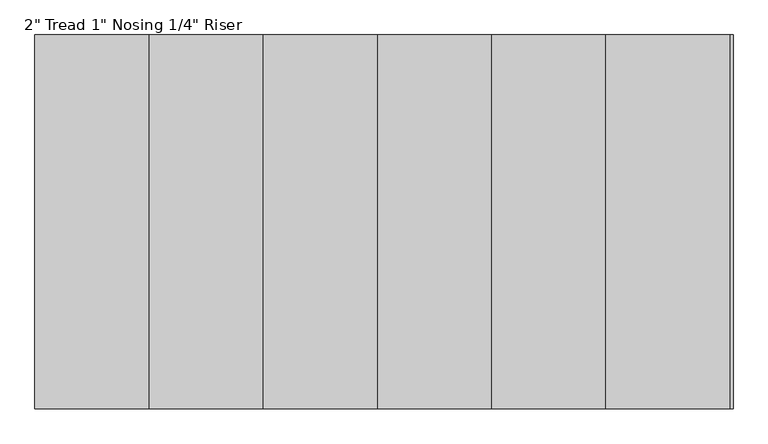
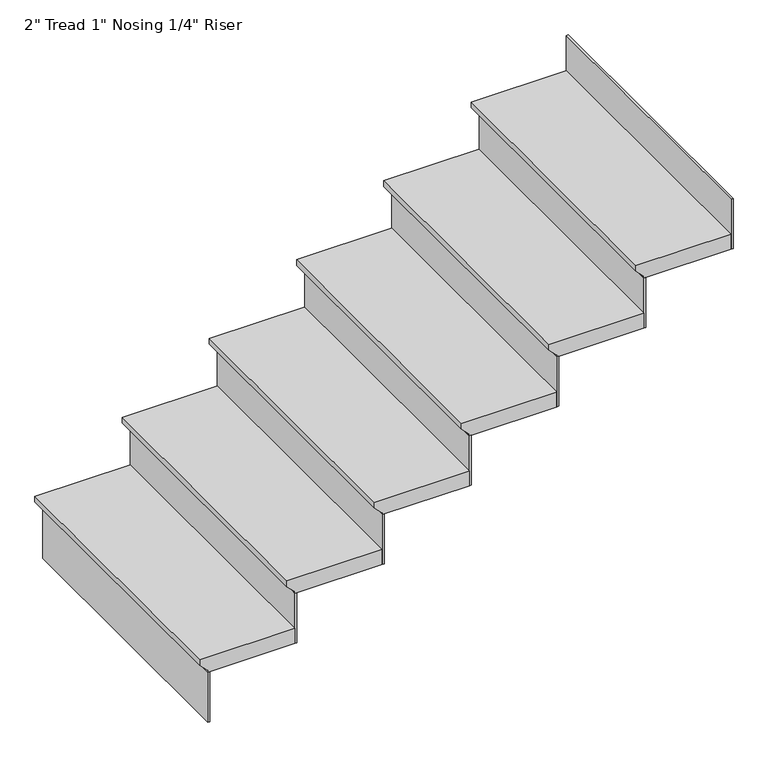
"""IFC4 building model written with IfcOpenShell, lengths in millimetres: stair flight geometry."""

from ifc_helpers import new_model, si_unit, frame, origin, place, context, project, spatial, polyline, outline, extrude, source, transform, mapped, element, save


def stair_flight_86d1b198(model_context):
    return source(origin(), model_context, "Body", "SweptSolid", [
        extrude(outline(polyline([(2336.8, -8480.0517085), (2336.8, -8784.8517085), (2317.75, -8784.8517085), (2292.35, -8759.4517085), (2286.0, -8759.4517085), (2286.0, -8480.0517085), (2336.8, -8480.0517085)])), frame((0.0, 792.0165128, 0.0), z_axis=(0.0, 1.0, 0.0), x_axis=(0.0, 0.0, 1.0)), (0.0, 0.0, 1.0), 914.4),
        extrude(outline(polyline([(-8753.1017085, 792.0165128), (-8759.4517085, 792.0165128), (-8759.4517085, 1706.4165128), (-8753.1017085, 1706.4165128), (-8753.1017085, 792.0165128)])), frame((0.0, 0.0, 2116.6666667), z_axis=(0.0, 0.0, 1.0), x_axis=(1.0, 0.0, 0.0)), (0.0, 0.0, 1.0), 169.3333333),
        extrude(outline(polyline([(-8473.7017085, 792.0165128), (-8480.0517085, 792.0165128), (-8480.0517085, 1706.4165128), (-8473.7017085, 1706.4165128), (-8473.7017085, 792.0165128)])), frame((0.0, 0.0, 2286.0), z_axis=(0.0, 0.0, 1.0), x_axis=(1.0, 0.0, 0.0)), (0.0, 0.0, 1.0), 169.3333333),
        extrude(outline(polyline([(2506.1333333, -8200.6517085), (2506.1333333, -8505.4517085), (2487.0833333, -8505.4517085), (2461.6833333, -8480.0517085), (2455.3333333, -8480.0517085), (2455.3333333, -8200.6517085), (2506.1333333, -8200.6517085)])), frame((0.0, 792.0165128, 0.0), z_axis=(0.0, 1.0, 0.0), x_axis=(0.0, 0.0, 1.0)), (0.0, 0.0, 1.0), 914.4),
        extrude(outline(polyline([(-8194.3017085, 792.0165128), (-8200.6517085, 792.0165128), (-8200.6517085, 1706.4165128), (-8194.3017085, 1706.4165128), (-8194.3017085, 792.0165128)])), frame((0.0, 0.0, 2455.3333333), z_axis=(0.0, 0.0, 1.0), x_axis=(1.0, 0.0, 0.0)), (0.0, 0.0, 1.0), 169.3333333),
        extrude(outline(polyline([(2675.4666667, -7921.2517085), (2675.4666667, -8226.0517085), (2656.4166667, -8226.0517085), (2631.0166667, -8200.6517085), (2624.6666667, -8200.6517085), (2624.6666667, -7921.2517085), (2675.4666667, -7921.2517085)])), frame((0.0, 792.0165128, 0.0), z_axis=(0.0, 1.0, 0.0), x_axis=(0.0, 0.0, 1.0)), (0.0, 0.0, 1.0), 914.4),
        extrude(outline(polyline([(-7914.9017085, 792.0165128), (-7921.2517085, 792.0165128), (-7921.2517085, 1706.4165128), (-7914.9017085, 1706.4165128), (-7914.9017085, 792.0165128)])), frame((0.0, 0.0, 2624.6666667), z_axis=(0.0, 0.0, 1.0), x_axis=(1.0, 0.0, 0.0)), (0.0, 0.0, 1.0), 169.3333333),
        extrude(outline(polyline([(2844.8, -7641.8517085), (2844.8, -7946.6517085), (2825.75, -7946.6517085), (2800.35, -7921.2517085), (2794.0, -7921.2517085), (2794.0, -7641.8517085), (2844.8, -7641.8517085)])), frame((0.0, 792.0165128, 0.0), z_axis=(0.0, 1.0, 0.0), x_axis=(0.0, 0.0, 1.0)), (0.0, 0.0, 1.0), 914.4),
        extrude(outline(polyline([(-7635.5017085, 792.0165128), (-7641.8517085, 792.0165128), (-7641.8517085, 1706.4165128), (-7635.5017085, 1706.4165128), (-7635.5017085, 792.0165128)])), frame((0.0, 0.0, 2794.0), z_axis=(0.0, 0.0, 1.0), x_axis=(1.0, 0.0, 0.0)), (0.0, 0.0, 1.0), 169.3333333),
        extrude(outline(polyline([(3014.1333333, -7362.4517085), (3014.1333333, -7667.2517085), (2995.0833333, -7667.2517085), (2969.6833333, -7641.8517085), (2963.3333333, -7641.8517085), (2963.3333333, -7362.4517085), (3014.1333333, -7362.4517085)])), frame((0.0, 792.0165128, 0.0), z_axis=(0.0, 1.0, 0.0), x_axis=(0.0, 0.0, 1.0)), (0.0, 0.0, 1.0), 914.4),
        extrude(outline(polyline([(-7356.1017085, 792.0165128), (-7362.4517085, 792.0165128), (-7362.4517085, 1706.4165128), (-7356.1017085, 1706.4165128), (-7356.1017085, 792.0165128)])), frame((0.0, 0.0, 2963.3333333), z_axis=(0.0, 0.0, 1.0), x_axis=(1.0, 0.0, 0.0)), (0.0, 0.0, 1.0), 169.3333333),
        extrude(outline(polyline([(-7076.7017085, 792.0165128), (-7083.0517085, 792.0165128), (-7083.0517085, 1706.4165128), (-7076.7017085, 1706.4165128), (-7076.7017085, 792.0165128)])), frame((0.0, 0.0, 3132.6666667), z_axis=(0.0, 0.0, 1.0), x_axis=(1.0, 0.0, 0.0)), (0.0, 0.0, 1.0), 169.3333333),
        extrude(outline(polyline([(3183.4666667, -7083.0517085), (3183.4666667, -7387.8517085), (3164.4166667, -7387.8517085), (3139.0166667, -7362.4517085), (3132.6666667, -7362.4517085), (3132.6666667, -7083.0517085), (3183.4666667, -7083.0517085)])), frame((0.0, 792.0165128, 0.0), z_axis=(0.0, 1.0, 0.0), x_axis=(0.0, 0.0, 1.0)), (0.0, 0.0, 1.0), 914.4),
    ])


if __name__ == "__main__":
    model = new_model("IFC4")
    model_context = context("Model", 3, world=origin())
    ifc_project = project(units=[si_unit("LENGTHUNIT", "METRE", prefix="MILLI")], contexts=[model_context])
    site = spatial("IfcSite", under=ifc_project)
    building = spatial("IfcBuilding", under=site)
    placement = place(None, origin())
    stair_flight_shape = stair_flight_86d1b198(model_context)
    element("IfcStairFlight", 1, ObjectType="2\" Tread 1\" Nosing 1/4\" Riser", at=placement, inside=building, context=model_context, shape_type="MappedRepresentation", body=[
        mapped(stair_flight_shape, transform((0.0, 0.0, 0.0), x_axis=(1.0, 0.0, 0.0), y_axis=(0.0, 1.0, 0.0), z_axis=(0.0, 0.0, 1.0))),
    ])
    save(model, "model.ifc")
